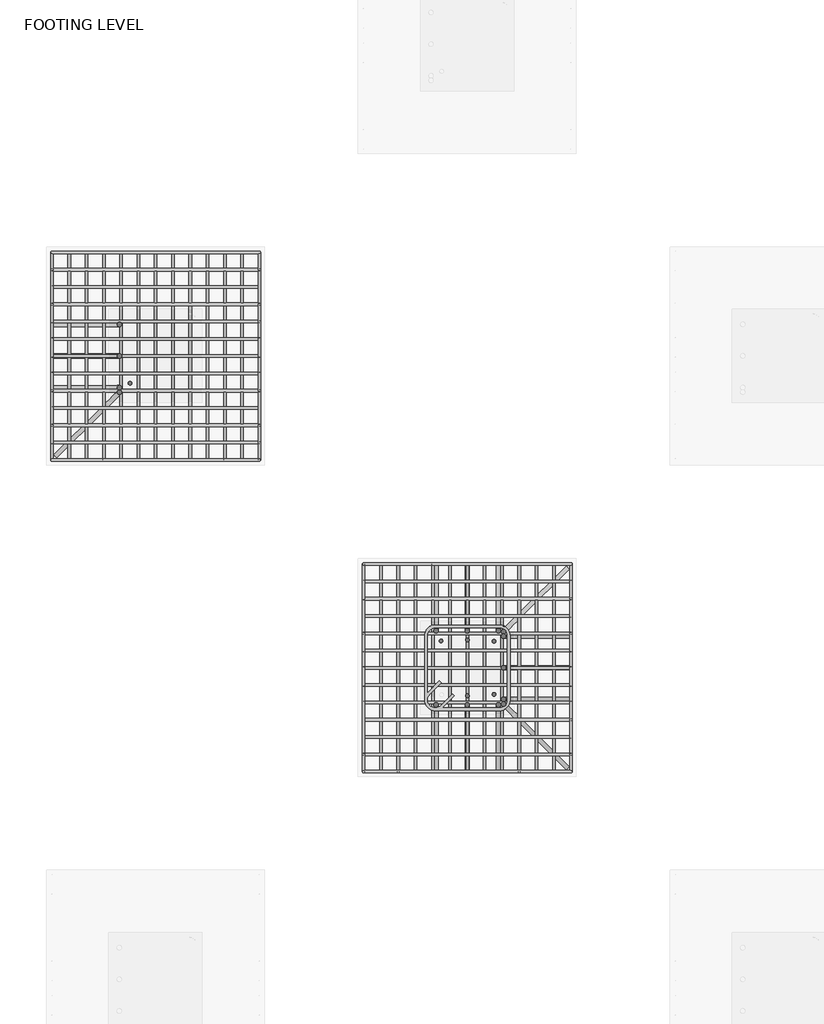
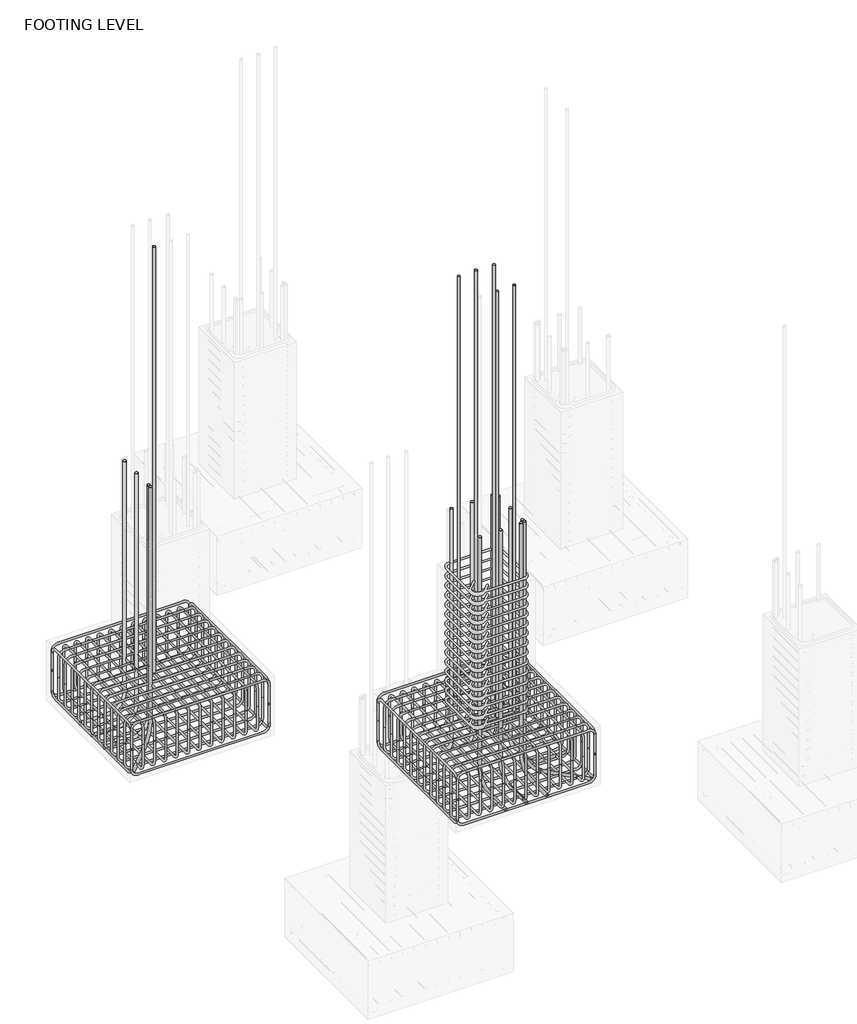
# One storey, part 4 of 10: 23 reinforcing bars.
"""IFC4 building model written with IfcOpenShell, lengths in millimetres."""

from ifc_helpers import new_model, si_unit, point, frame, origin, place, context, project, spatial, polyline, circle_curve, trimmed, segment, composite_curve, source, transform, mapped, element, save
from ifc_brep_helpers import swept_disk

model = new_model("IFC4")

# Units and contexts
model_context = context("Model", 3, world=origin())
ifc_project = project(units=[si_unit("LENGTHUNIT", "METRE", prefix="MILLI")], contexts=[model_context])

# Site, building, storey
site = spatial("IfcSite", under=ifc_project)
building = spatial("IfcBuilding", under=site)
storey = spatial("IfcBuildingStorey", under=building, Name="FOOTING LEVEL", Elevation=-2133.6)

# Reinforcing bars
placement = place(None, origin())
reinforcing_bar_shape = source(origin(), model_context, "Body", "SolidModel", [
    swept_disk(composite_curve([segment(polyline([(-11826.9269037, 6852.4829396, -2583.0), (-11826.9269037, 6852.4829396, -2905.1)]), True, "CONTINUOUS"), segment(trimmed(circle_curve(frame((-11917.1269037, 6852.4829396, -2905.1), z_axis=(0.0, 1.0, 0.0), x_axis=(90.20000000000073, 0.0, 0.0)), 90.2), [point((-11826.9269037, 6852.4829396, -2905.1))], [point((-11917.1269037, 6852.4829396, -2995.3))], True, "CARTESIAN"), True, "CONTINUOUS"), segment(polyline([(-11917.1269037, 6852.4829396, -2995.3), (-13764.9269037, 6852.4829396, -2995.3)]), True, "CONTINUOUS"), segment(trimmed(circle_curve(frame((-13764.9269037, 6852.4829396, -2905.1), z_axis=(0.0, 1.0, 0.0), x_axis=(0.0, 0.0, -90.20000000000027)), 90.2), [point((-13764.9269037, 6852.4829396, -2995.3))], [point((-13855.1269037, 6852.4829396, -2905.1))], True, "CARTESIAN"), True, "CONTINUOUS"), segment(polyline([(-13855.1269037, 6852.4829396, -2905.1), (-13855.1269037, 6852.4829396, -2583.0)]), True, "CONTINUOUS")], self_intersect=False), 12.7),
])
element("IfcReinforcingBar", 1, at=placement, inside=storey, context=model_context, shape_type="MappedRepresentation", body=[
    mapped(reinforcing_bar_shape, transform((0.0, 0.0, 0.0), x_axis=(1.0, 0.0, 0.0), y_axis=(0.0, 1.0, 0.0), z_axis=(0.0, 0.0, 1.0))),
    mapped(reinforcing_bar_shape, transform((0.0, -169.0166667, 0.0), x_axis=(1.0, 0.0, 0.0), y_axis=(0.0, 1.0, 0.0), z_axis=(0.0, 0.0, 1.0))),
    mapped(reinforcing_bar_shape, transform((0.0, -338.0333333, 0.0), x_axis=(1.0, 0.0, 0.0), y_axis=(0.0, 1.0, 0.0), z_axis=(0.0, 0.0, 1.0))),
    mapped(reinforcing_bar_shape, transform((0.0, -507.05, 0.0), x_axis=(1.0, 0.0, 0.0), y_axis=(0.0, 1.0, 0.0), z_axis=(0.0, 0.0, 1.0))),
    mapped(reinforcing_bar_shape, transform((0.0, -676.0666667, 0.0), x_axis=(1.0, 0.0, 0.0), y_axis=(0.0, 1.0, 0.0), z_axis=(0.0, 0.0, 1.0))),
    mapped(reinforcing_bar_shape, transform((0.0, -845.0833333, 0.0), x_axis=(1.0, 0.0, 0.0), y_axis=(0.0, 1.0, 0.0), z_axis=(0.0, 0.0, 1.0))),
    mapped(reinforcing_bar_shape, transform((0.0, -1014.1, 0.0), x_axis=(1.0, 0.0, 0.0), y_axis=(0.0, 1.0, 0.0), z_axis=(0.0, 0.0, 1.0))),
    mapped(reinforcing_bar_shape, transform((0.0, -1183.1166667, 0.0), x_axis=(1.0, 0.0, 0.0), y_axis=(0.0, 1.0, 0.0), z_axis=(0.0, 0.0, 1.0))),
    mapped(reinforcing_bar_shape, transform((0.0, -1352.1333333, 0.0), x_axis=(1.0, 0.0, 0.0), y_axis=(0.0, 1.0, 0.0), z_axis=(0.0, 0.0, 1.0))),
    mapped(reinforcing_bar_shape, transform((0.0, -1521.15, 0.0), x_axis=(1.0, 0.0, 0.0), y_axis=(0.0, 1.0, 0.0), z_axis=(0.0, 0.0, 1.0))),
    mapped(reinforcing_bar_shape, transform((0.0, -1690.1666667, 0.0), x_axis=(1.0, 0.0, 0.0), y_axis=(0.0, 1.0, 0.0), z_axis=(0.0, 0.0, 1.0))),
    mapped(reinforcing_bar_shape, transform((0.0, -1859.1833333, 0.0), x_axis=(1.0, 0.0, 0.0), y_axis=(0.0, 1.0, 0.0), z_axis=(0.0, 0.0, 1.0))),
    mapped(reinforcing_bar_shape, transform((0.0, -2028.2, 0.0), x_axis=(1.0, 0.0, 0.0), y_axis=(0.0, 1.0, 0.0), z_axis=(0.0, 0.0, 1.0))),
])
reinforcing_bar_2_shape = source(origin(), model_context, "Body", "SolidModel", [
    swept_disk(composite_curve([segment(polyline([(-13855.1269037, 6852.4829396, -2598.6), (-13855.1269037, 6852.4829396, -2276.5)]), True, "CONTINUOUS"), segment(trimmed(circle_curve(frame((-13764.9269037, 6852.4829396, -2276.5), z_axis=(0.0, 1.0, 0.0), x_axis=(-90.20000000000073, 0.0, 0.0)), 90.2), [point((-13855.1269037, 6852.4829396, -2276.5))], [point((-13764.9269037, 6852.4829396, -2186.3))], True, "CARTESIAN"), True, "CONTINUOUS"), segment(polyline([(-13764.9269037, 6852.4829396, -2186.3), (-11917.1269037, 6852.4829396, -2186.3)]), True, "CONTINUOUS"), segment(trimmed(circle_curve(frame((-11917.1269037, 6852.4829396, -2276.5), z_axis=(0.0, 1.0, 0.0), x_axis=(0.0, 0.0, 90.19999999999982)), 90.2), [point((-11917.1269037, 6852.4829396, -2186.3))], [point((-11826.9269037, 6852.4829396, -2276.5))], True, "CARTESIAN"), True, "CONTINUOUS"), segment(polyline([(-11826.9269037, 6852.4829396, -2276.5), (-11826.9269037, 6852.4829396, -2598.6)]), True, "CONTINUOUS")], self_intersect=False), 12.7),
])
element("IfcReinforcingBar", 2, at=placement, inside=storey, context=model_context, shape_type="MappedRepresentation", body=[
    mapped(reinforcing_bar_2_shape, transform((0.0, 0.0, 0.0), x_axis=(1.0, 0.0, 0.0), y_axis=(0.0, 1.0, 0.0), z_axis=(0.0, 0.0, 1.0))),
    mapped(reinforcing_bar_2_shape, transform((0.0, -169.0166667, 0.0), x_axis=(1.0, 0.0, 0.0), y_axis=(0.0, 1.0, 0.0), z_axis=(0.0, 0.0, 1.0))),
    mapped(reinforcing_bar_2_shape, transform((0.0, -338.0333333, 0.0), x_axis=(1.0, 0.0, 0.0), y_axis=(0.0, 1.0, 0.0), z_axis=(0.0, 0.0, 1.0))),
    mapped(reinforcing_bar_2_shape, transform((0.0, -507.05, 0.0), x_axis=(1.0, 0.0, 0.0), y_axis=(0.0, 1.0, 0.0), z_axis=(0.0, 0.0, 1.0))),
    mapped(reinforcing_bar_2_shape, transform((0.0, -676.0666667, 0.0), x_axis=(1.0, 0.0, 0.0), y_axis=(0.0, 1.0, 0.0), z_axis=(0.0, 0.0, 1.0))),
    mapped(reinforcing_bar_2_shape, transform((0.0, -845.0833333, 0.0), x_axis=(1.0, 0.0, 0.0), y_axis=(0.0, 1.0, 0.0), z_axis=(0.0, 0.0, 1.0))),
    mapped(reinforcing_bar_2_shape, transform((0.0, -1014.1, 0.0), x_axis=(1.0, 0.0, 0.0), y_axis=(0.0, 1.0, 0.0), z_axis=(0.0, 0.0, 1.0))),
    mapped(reinforcing_bar_2_shape, transform((0.0, -1183.1166667, 0.0), x_axis=(1.0, 0.0, 0.0), y_axis=(0.0, 1.0, 0.0), z_axis=(0.0, 0.0, 1.0))),
    mapped(reinforcing_bar_2_shape, transform((0.0, -1352.1333333, 0.0), x_axis=(1.0, 0.0, 0.0), y_axis=(0.0, 1.0, 0.0), z_axis=(0.0, 0.0, 1.0))),
    mapped(reinforcing_bar_2_shape, transform((0.0, -1521.15, 0.0), x_axis=(1.0, 0.0, 0.0), y_axis=(0.0, 1.0, 0.0), z_axis=(0.0, 0.0, 1.0))),
    mapped(reinforcing_bar_2_shape, transform((0.0, -1690.1666667, 0.0), x_axis=(1.0, 0.0, 0.0), y_axis=(0.0, 1.0, 0.0), z_axis=(0.0, 0.0, 1.0))),
    mapped(reinforcing_bar_2_shape, transform((0.0, -1859.1833333, 0.0), x_axis=(1.0, 0.0, 0.0), y_axis=(0.0, 1.0, 0.0), z_axis=(0.0, 0.0, 1.0))),
    mapped(reinforcing_bar_2_shape, transform((0.0, -2028.2, 0.0), x_axis=(1.0, 0.0, 0.0), y_axis=(0.0, 1.0, 0.0), z_axis=(0.0, 0.0, 1.0))),
])
reinforcing_bar_3_shape = source(origin(), model_context, "Body", "SolidModel", [
    swept_disk(composite_curve([segment(polyline([(-11826.9269037, 4824.2829396, -2559.4978077), (-11826.9269037, 4824.2829396, -2881.5978077)]), True, "CONTINUOUS"), segment(trimmed(circle_curve(frame((-11826.9269037, 4914.4829396, -2881.5978077), z_axis=(1.0, 0.0, 0.0), x_axis=(0.0, -90.19999999999982, 0.0)), 90.2), [point((-11826.9269037, 4824.2829396, -2881.5978077))], [point((-11826.9269037, 4914.4829396, -2971.7978077))], True, "CARTESIAN"), True, "CONTINUOUS"), segment(polyline([(-11826.9269037, 4914.4829396, -2971.7978077), (-11826.9269037, 6762.2829396, -2971.7978077)]), True, "CONTINUOUS"), segment(trimmed(circle_curve(frame((-11826.9269037, 6762.2829396, -2881.5978077), z_axis=(1.0, 0.0, 0.0), x_axis=(0.0, 0.0, -90.19999999999982)), 90.2), [point((-11826.9269037, 6762.2829396, -2971.7978077))], [point((-11826.9269037, 6852.4829396, -2881.5978077))], True, "CARTESIAN"), True, "CONTINUOUS"), segment(polyline([(-11826.9269037, 6852.4829396, -2881.5978077), (-11826.9269037, 6852.4829396, -2559.4978077)]), True, "CONTINUOUS")], self_intersect=False), 12.7),
])
element("IfcReinforcingBar", 3, at=placement, inside=storey, context=model_context, shape_type="MappedRepresentation", body=[
    mapped(reinforcing_bar_3_shape, transform((0.0, 0.0, 0.0), x_axis=(1.0, 0.0, 0.0), y_axis=(0.0, 1.0, 0.0), z_axis=(0.0, 0.0, 1.0))),
    mapped(reinforcing_bar_3_shape, transform((-169.0166667, 0.0, 0.0), x_axis=(1.0, 0.0, 0.0), y_axis=(0.0, 1.0, 0.0), z_axis=(0.0, 0.0, 1.0))),
    mapped(reinforcing_bar_3_shape, transform((-338.0333333, 0.0, 0.0), x_axis=(1.0, 0.0, 0.0), y_axis=(0.0, 1.0, 0.0), z_axis=(0.0, 0.0, 1.0))),
    mapped(reinforcing_bar_3_shape, transform((-507.05, 0.0, 0.0), x_axis=(1.0, 0.0, 0.0), y_axis=(0.0, 1.0, 0.0), z_axis=(0.0, 0.0, 1.0))),
    mapped(reinforcing_bar_3_shape, transform((-676.0666667, 0.0, 0.0), x_axis=(1.0, 0.0, 0.0), y_axis=(0.0, 1.0, 0.0), z_axis=(0.0, 0.0, 1.0))),
    mapped(reinforcing_bar_3_shape, transform((-845.0833333, 0.0, 0.0), x_axis=(1.0, 0.0, 0.0), y_axis=(0.0, 1.0, 0.0), z_axis=(0.0, 0.0, 1.0))),
    mapped(reinforcing_bar_3_shape, transform((-1014.1, 0.0, 0.0), x_axis=(1.0, 0.0, 0.0), y_axis=(0.0, 1.0, 0.0), z_axis=(0.0, 0.0, 1.0))),
    mapped(reinforcing_bar_3_shape, transform((-1183.1166667, 0.0, 0.0), x_axis=(1.0, 0.0, 0.0), y_axis=(0.0, 1.0, 0.0), z_axis=(0.0, 0.0, 1.0))),
    mapped(reinforcing_bar_3_shape, transform((-1352.1333333, 0.0, 0.0), x_axis=(1.0, 0.0, 0.0), y_axis=(0.0, 1.0, 0.0), z_axis=(0.0, 0.0, 1.0))),
    mapped(reinforcing_bar_3_shape, transform((-1521.15, 0.0, 0.0), x_axis=(1.0, 0.0, 0.0), y_axis=(0.0, 1.0, 0.0), z_axis=(0.0, 0.0, 1.0))),
    mapped(reinforcing_bar_3_shape, transform((-1690.1666667, 0.0, 0.0), x_axis=(1.0, 0.0, 0.0), y_axis=(0.0, 1.0, 0.0), z_axis=(0.0, 0.0, 1.0))),
    mapped(reinforcing_bar_3_shape, transform((-1859.1833333, 0.0, 0.0), x_axis=(1.0, 0.0, 0.0), y_axis=(0.0, 1.0, 0.0), z_axis=(0.0, 0.0, 1.0))),
    mapped(reinforcing_bar_3_shape, transform((-2028.2, 0.0, 0.0), x_axis=(1.0, 0.0, 0.0), y_axis=(0.0, 1.0, 0.0), z_axis=(0.0, 0.0, 1.0))),
])
reinforcing_bar_4_shape = source(origin(), model_context, "Body", "SolidModel", [
    swept_disk(composite_curve([segment(polyline([(-13855.1269037, 4824.2829396, -2622.9919875), (-13855.1269037, 4824.2829396, -2300.8919875)]), True, "CONTINUOUS"), segment(trimmed(circle_curve(frame((-13855.1269037, 4914.4829396, -2300.8919875), z_axis=(-1.0, 0.0, 0.0), x_axis=(0.0, -90.19999999999982, 0.0)), 90.2), [point((-13855.1269037, 4824.2829396, -2300.8919875))], [point((-13855.1269037, 4914.4829396, -2210.6919875))], True, "CARTESIAN"), True, "CONTINUOUS"), segment(polyline([(-13855.1269037, 4914.4829396, -2210.6919875), (-13855.1269037, 6762.2829396, -2210.6919875)]), True, "CONTINUOUS"), segment(trimmed(circle_curve(frame((-13855.1269037, 6762.2829396, -2300.8919875), z_axis=(-1.0, 0.0, 0.0), x_axis=(0.0, 0.0, 90.20000000000027)), 90.2), [point((-13855.1269037, 6762.2829396, -2210.6919875))], [point((-13855.1269037, 6852.4829396, -2300.8919875))], True, "CARTESIAN"), True, "CONTINUOUS"), segment(polyline([(-13855.1269037, 6852.4829396, -2300.8919875), (-13855.1269037, 6852.4829396, -2622.9919875)]), True, "CONTINUOUS")], self_intersect=False), 12.7),
])
element("IfcReinforcingBar", 4, at=placement, inside=storey, context=model_context, shape_type="MappedRepresentation", body=[
    mapped(reinforcing_bar_4_shape, transform((0.0, 0.0, 0.0), x_axis=(1.0, 0.0, 0.0), y_axis=(0.0, 1.0, 0.0), z_axis=(0.0, 0.0, 1.0))),
    mapped(reinforcing_bar_4_shape, transform((169.0166667, 0.0, 0.0), x_axis=(1.0, 0.0, 0.0), y_axis=(0.0, 1.0, 0.0), z_axis=(0.0, 0.0, 1.0))),
    mapped(reinforcing_bar_4_shape, transform((338.0333333, 0.0, 0.0), x_axis=(1.0, 0.0, 0.0), y_axis=(0.0, 1.0, 0.0), z_axis=(0.0, 0.0, 1.0))),
    mapped(reinforcing_bar_4_shape, transform((507.05, 0.0, 0.0), x_axis=(1.0, 0.0, 0.0), y_axis=(0.0, 1.0, 0.0), z_axis=(0.0, 0.0, 1.0))),
    mapped(reinforcing_bar_4_shape, transform((676.0666667, 0.0, 0.0), x_axis=(1.0, 0.0, 0.0), y_axis=(0.0, 1.0, 0.0), z_axis=(0.0, 0.0, 1.0))),
    mapped(reinforcing_bar_4_shape, transform((845.0833333, 0.0, 0.0), x_axis=(1.0, 0.0, 0.0), y_axis=(0.0, 1.0, 0.0), z_axis=(0.0, 0.0, 1.0))),
    mapped(reinforcing_bar_4_shape, transform((1014.1, 0.0, 0.0), x_axis=(1.0, 0.0, 0.0), y_axis=(0.0, 1.0, 0.0), z_axis=(0.0, 0.0, 1.0))),
    mapped(reinforcing_bar_4_shape, transform((1183.1166667, 0.0, 0.0), x_axis=(1.0, 0.0, 0.0), y_axis=(0.0, 1.0, 0.0), z_axis=(0.0, 0.0, 1.0))),
    mapped(reinforcing_bar_4_shape, transform((1352.1333333, 0.0, 0.0), x_axis=(1.0, 0.0, 0.0), y_axis=(0.0, 1.0, 0.0), z_axis=(0.0, 0.0, 1.0))),
    mapped(reinforcing_bar_4_shape, transform((1521.15, 0.0, 0.0), x_axis=(1.0, 0.0, 0.0), y_axis=(0.0, 1.0, 0.0), z_axis=(0.0, 0.0, 1.0))),
    mapped(reinforcing_bar_4_shape, transform((1690.1666667, 0.0, 0.0), x_axis=(1.0, 0.0, 0.0), y_axis=(0.0, 1.0, 0.0), z_axis=(0.0, 0.0, 1.0))),
    mapped(reinforcing_bar_4_shape, transform((1859.1833333, 0.0, 0.0), x_axis=(1.0, 0.0, 0.0), y_axis=(0.0, 1.0, 0.0), z_axis=(0.0, 0.0, 1.0))),
    mapped(reinforcing_bar_4_shape, transform((2028.2, 0.0, 0.0), x_axis=(1.0, 0.0, 0.0), y_axis=(0.0, 1.0, 0.0), z_axis=(0.0, 0.0, 1.0))),
])
reinforcing_bar_5_shape = source(origin(), model_context, "Body", "SolidModel", [
    swept_disk(composite_curve([segment(polyline([(-8778.9269037, 3804.4829396, -2583.0), (-8778.9269037, 3804.4829396, -2905.1)]), True, "CONTINUOUS"), segment(trimmed(circle_curve(frame((-8869.1269037, 3804.4829396, -2905.1), z_axis=(0.0, 1.0, 0.0), x_axis=(90.20000000000073, 0.0, 0.0)), 90.2), [point((-8778.9269037, 3804.4829396, -2905.1))], [point((-8869.1269037, 3804.4829396, -2995.3))], True, "CARTESIAN"), True, "CONTINUOUS"), segment(polyline([(-8869.1269037, 3804.4829396, -2995.3), (-10716.9269037, 3804.4829396, -2995.3)]), True, "CONTINUOUS"), segment(trimmed(circle_curve(frame((-10716.9269037, 3804.4829396, -2905.1), z_axis=(0.0, 1.0, 0.0), x_axis=(0.0, 0.0, -90.20000000000027)), 90.2), [point((-10716.9269037, 3804.4829396, -2995.3))], [point((-10807.1269037, 3804.4829396, -2905.1))], True, "CARTESIAN"), True, "CONTINUOUS"), segment(polyline([(-10807.1269037, 3804.4829396, -2905.1), (-10807.1269037, 3804.4829396, -2583.0)]), True, "CONTINUOUS")], self_intersect=False), 12.7),
])
element("IfcReinforcingBar", 5, at=placement, inside=storey, context=model_context, shape_type="MappedRepresentation", body=[
    mapped(reinforcing_bar_5_shape, transform((0.0, 0.0, 0.0), x_axis=(1.0, 0.0, 0.0), y_axis=(0.0, 1.0, 0.0), z_axis=(0.0, 0.0, 1.0))),
    mapped(reinforcing_bar_5_shape, transform((0.0, -169.0166667, 0.0), x_axis=(1.0, 0.0, 0.0), y_axis=(0.0, 1.0, 0.0), z_axis=(0.0, 0.0, 1.0))),
    mapped(reinforcing_bar_5_shape, transform((0.0, -338.0333333, 0.0), x_axis=(1.0, 0.0, 0.0), y_axis=(0.0, 1.0, 0.0), z_axis=(0.0, 0.0, 1.0))),
    mapped(reinforcing_bar_5_shape, transform((0.0, -507.05, 0.0), x_axis=(1.0, 0.0, 0.0), y_axis=(0.0, 1.0, 0.0), z_axis=(0.0, 0.0, 1.0))),
    mapped(reinforcing_bar_5_shape, transform((0.0, -676.0666667, 0.0), x_axis=(1.0, 0.0, 0.0), y_axis=(0.0, 1.0, 0.0), z_axis=(0.0, 0.0, 1.0))),
    mapped(reinforcing_bar_5_shape, transform((0.0, -845.0833333, 0.0), x_axis=(1.0, 0.0, 0.0), y_axis=(0.0, 1.0, 0.0), z_axis=(0.0, 0.0, 1.0))),
    mapped(reinforcing_bar_5_shape, transform((0.0, -1014.1, 0.0), x_axis=(1.0, 0.0, 0.0), y_axis=(0.0, 1.0, 0.0), z_axis=(0.0, 0.0, 1.0))),
    mapped(reinforcing_bar_5_shape, transform((0.0, -1183.1166667, 0.0), x_axis=(1.0, 0.0, 0.0), y_axis=(0.0, 1.0, 0.0), z_axis=(0.0, 0.0, 1.0))),
    mapped(reinforcing_bar_5_shape, transform((0.0, -1352.1333333, 0.0), x_axis=(1.0, 0.0, 0.0), y_axis=(0.0, 1.0, 0.0), z_axis=(0.0, 0.0, 1.0))),
    mapped(reinforcing_bar_5_shape, transform((0.0, -1521.15, 0.0), x_axis=(1.0, 0.0, 0.0), y_axis=(0.0, 1.0, 0.0), z_axis=(0.0, 0.0, 1.0))),
    mapped(reinforcing_bar_5_shape, transform((0.0, -1690.1666667, 0.0), x_axis=(1.0, 0.0, 0.0), y_axis=(0.0, 1.0, 0.0), z_axis=(0.0, 0.0, 1.0))),
    mapped(reinforcing_bar_5_shape, transform((0.0, -1859.1833333, 0.0), x_axis=(1.0, 0.0, 0.0), y_axis=(0.0, 1.0, 0.0), z_axis=(0.0, 0.0, 1.0))),
    mapped(reinforcing_bar_5_shape, transform((0.0, -2028.2, 0.0), x_axis=(1.0, 0.0, 0.0), y_axis=(0.0, 1.0, 0.0), z_axis=(0.0, 0.0, 1.0))),
])
reinforcing_bar_6_shape = source(origin(), model_context, "Body", "SolidModel", [
    swept_disk(composite_curve([segment(polyline([(-10807.1269037, 3804.4829396, -2598.6), (-10807.1269037, 3804.4829396, -2276.5)]), True, "CONTINUOUS"), segment(trimmed(circle_curve(frame((-10716.9269037, 3804.4829396, -2276.5), z_axis=(0.0, 1.0, 0.0), x_axis=(-90.20000000000073, 0.0, 0.0)), 90.2), [point((-10807.1269037, 3804.4829396, -2276.5))], [point((-10716.9269037, 3804.4829396, -2186.3))], True, "CARTESIAN"), True, "CONTINUOUS"), segment(polyline([(-10716.9269037, 3804.4829396, -2186.3), (-8869.1269037, 3804.4829396, -2186.3)]), True, "CONTINUOUS"), segment(trimmed(circle_curve(frame((-8869.1269037, 3804.4829396, -2276.5), z_axis=(0.0, 1.0, 0.0), x_axis=(0.0, 0.0, 90.19999999999982)), 90.2), [point((-8869.1269037, 3804.4829396, -2186.3))], [point((-8778.9269037, 3804.4829396, -2276.5))], True, "CARTESIAN"), True, "CONTINUOUS"), segment(polyline([(-8778.9269037, 3804.4829396, -2276.5), (-8778.9269037, 3804.4829396, -2598.6)]), True, "CONTINUOUS")], self_intersect=False), 12.7),
])
element("IfcReinforcingBar", 6, at=placement, inside=storey, context=model_context, shape_type="MappedRepresentation", body=[
    mapped(reinforcing_bar_6_shape, transform((0.0, 0.0, 0.0), x_axis=(1.0, 0.0, 0.0), y_axis=(0.0, 1.0, 0.0), z_axis=(0.0, 0.0, 1.0))),
    mapped(reinforcing_bar_6_shape, transform((0.0, -169.0166667, 0.0), x_axis=(1.0, 0.0, 0.0), y_axis=(0.0, 1.0, 0.0), z_axis=(0.0, 0.0, 1.0))),
    mapped(reinforcing_bar_6_shape, transform((0.0, -338.0333333, 0.0), x_axis=(1.0, 0.0, 0.0), y_axis=(0.0, 1.0, 0.0), z_axis=(0.0, 0.0, 1.0))),
    mapped(reinforcing_bar_6_shape, transform((0.0, -507.05, 0.0), x_axis=(1.0, 0.0, 0.0), y_axis=(0.0, 1.0, 0.0), z_axis=(0.0, 0.0, 1.0))),
    mapped(reinforcing_bar_6_shape, transform((0.0, -676.0666667, 0.0), x_axis=(1.0, 0.0, 0.0), y_axis=(0.0, 1.0, 0.0), z_axis=(0.0, 0.0, 1.0))),
    mapped(reinforcing_bar_6_shape, transform((0.0, -845.0833333, 0.0), x_axis=(1.0, 0.0, 0.0), y_axis=(0.0, 1.0, 0.0), z_axis=(0.0, 0.0, 1.0))),
    mapped(reinforcing_bar_6_shape, transform((0.0, -1014.1, 0.0), x_axis=(1.0, 0.0, 0.0), y_axis=(0.0, 1.0, 0.0), z_axis=(0.0, 0.0, 1.0))),
    mapped(reinforcing_bar_6_shape, transform((0.0, -1183.1166667, 0.0), x_axis=(1.0, 0.0, 0.0), y_axis=(0.0, 1.0, 0.0), z_axis=(0.0, 0.0, 1.0))),
    mapped(reinforcing_bar_6_shape, transform((0.0, -1352.1333333, 0.0), x_axis=(1.0, 0.0, 0.0), y_axis=(0.0, 1.0, 0.0), z_axis=(0.0, 0.0, 1.0))),
    mapped(reinforcing_bar_6_shape, transform((0.0, -1521.15, 0.0), x_axis=(1.0, 0.0, 0.0), y_axis=(0.0, 1.0, 0.0), z_axis=(0.0, 0.0, 1.0))),
    mapped(reinforcing_bar_6_shape, transform((0.0, -1690.1666667, 0.0), x_axis=(1.0, 0.0, 0.0), y_axis=(0.0, 1.0, 0.0), z_axis=(0.0, 0.0, 1.0))),
    mapped(reinforcing_bar_6_shape, transform((0.0, -1859.1833333, 0.0), x_axis=(1.0, 0.0, 0.0), y_axis=(0.0, 1.0, 0.0), z_axis=(0.0, 0.0, 1.0))),
    mapped(reinforcing_bar_6_shape, transform((0.0, -2028.2, 0.0), x_axis=(1.0, 0.0, 0.0), y_axis=(0.0, 1.0, 0.0), z_axis=(0.0, 0.0, 1.0))),
])
reinforcing_bar_7_shape = source(origin(), model_context, "Body", "SolidModel", [
    swept_disk(composite_curve([segment(polyline([(-8778.9269037, 1776.2829396, -2559.4978077), (-8778.9269037, 1776.2829396, -2881.5978077)]), True, "CONTINUOUS"), segment(trimmed(circle_curve(frame((-8778.9269037, 1866.4829396, -2881.5978077), z_axis=(1.0, 0.0, 0.0), x_axis=(0.0, -90.20000000000005, 0.0)), 90.2), [point((-8778.9269037, 1776.2829396, -2881.5978077))], [point((-8778.9269037, 1866.4829396, -2971.7978077))], True, "CARTESIAN"), True, "CONTINUOUS"), segment(polyline([(-8778.9269037, 1866.4829396, -2971.7978077), (-8778.9269037, 3714.2829396, -2971.7978077)]), True, "CONTINUOUS"), segment(trimmed(circle_curve(frame((-8778.9269037, 3714.2829396, -2881.5978077), z_axis=(1.0, 0.0, 0.0), x_axis=(0.0, 0.0, -90.19999999999982)), 90.2), [point((-8778.9269037, 3714.2829396, -2971.7978077))], [point((-8778.9269037, 3804.4829396, -2881.5978077))], True, "CARTESIAN"), True, "CONTINUOUS"), segment(polyline([(-8778.9269037, 3804.4829396, -2881.5978077), (-8778.9269037, 3804.4829396, -2559.4978077)]), True, "CONTINUOUS")], self_intersect=False), 12.7),
])
element("IfcReinforcingBar", 7, at=placement, inside=storey, context=model_context, shape_type="MappedRepresentation", body=[
    mapped(reinforcing_bar_7_shape, transform((0.0, 0.0, 0.0), x_axis=(1.0, 0.0, 0.0), y_axis=(0.0, 1.0, 0.0), z_axis=(0.0, 0.0, 1.0))),
    mapped(reinforcing_bar_7_shape, transform((-169.0166667, 0.0, 0.0), x_axis=(1.0, 0.0, 0.0), y_axis=(0.0, 1.0, 0.0), z_axis=(0.0, 0.0, 1.0))),
    mapped(reinforcing_bar_7_shape, transform((-338.0333333, 0.0, 0.0), x_axis=(1.0, 0.0, 0.0), y_axis=(0.0, 1.0, 0.0), z_axis=(0.0, 0.0, 1.0))),
    mapped(reinforcing_bar_7_shape, transform((-507.05, 0.0, 0.0), x_axis=(1.0, 0.0, 0.0), y_axis=(0.0, 1.0, 0.0), z_axis=(0.0, 0.0, 1.0))),
    mapped(reinforcing_bar_7_shape, transform((-676.0666667, 0.0, 0.0), x_axis=(1.0, 0.0, 0.0), y_axis=(0.0, 1.0, 0.0), z_axis=(0.0, 0.0, 1.0))),
    mapped(reinforcing_bar_7_shape, transform((-845.0833333, 0.0, 0.0), x_axis=(1.0, 0.0, 0.0), y_axis=(0.0, 1.0, 0.0), z_axis=(0.0, 0.0, 1.0))),
    mapped(reinforcing_bar_7_shape, transform((-1014.1, 0.0, 0.0), x_axis=(1.0, 0.0, 0.0), y_axis=(0.0, 1.0, 0.0), z_axis=(0.0, 0.0, 1.0))),
    mapped(reinforcing_bar_7_shape, transform((-1183.1166667, 0.0, 0.0), x_axis=(1.0, 0.0, 0.0), y_axis=(0.0, 1.0, 0.0), z_axis=(0.0, 0.0, 1.0))),
    mapped(reinforcing_bar_7_shape, transform((-1352.1333333, 0.0, 0.0), x_axis=(1.0, 0.0, 0.0), y_axis=(0.0, 1.0, 0.0), z_axis=(0.0, 0.0, 1.0))),
    mapped(reinforcing_bar_7_shape, transform((-1521.15, 0.0, 0.0), x_axis=(1.0, 0.0, 0.0), y_axis=(0.0, 1.0, 0.0), z_axis=(0.0, 0.0, 1.0))),
    mapped(reinforcing_bar_7_shape, transform((-1690.1666667, 0.0, 0.0), x_axis=(1.0, 0.0, 0.0), y_axis=(0.0, 1.0, 0.0), z_axis=(0.0, 0.0, 1.0))),
    mapped(reinforcing_bar_7_shape, transform((-1859.1833333, 0.0, 0.0), x_axis=(1.0, 0.0, 0.0), y_axis=(0.0, 1.0, 0.0), z_axis=(0.0, 0.0, 1.0))),
    mapped(reinforcing_bar_7_shape, transform((-2028.2, 0.0, 0.0), x_axis=(1.0, 0.0, 0.0), y_axis=(0.0, 1.0, 0.0), z_axis=(0.0, 0.0, 1.0))),
])
reinforcing_bar_8_shape = source(origin(), model_context, "Body", "SolidModel", [
    swept_disk(composite_curve([segment(polyline([(-10807.1269037, 1776.2829396, -2622.9919875), (-10807.1269037, 1776.2829396, -2300.8919875)]), True, "CONTINUOUS"), segment(trimmed(circle_curve(frame((-10807.1269037, 1866.4829396, -2300.8919875), z_axis=(-1.0, 0.0, 0.0), x_axis=(0.0, -90.20000000000005, 0.0)), 90.2), [point((-10807.1269037, 1776.2829396, -2300.8919875))], [point((-10807.1269037, 1866.4829396, -2210.6919875))], True, "CARTESIAN"), True, "CONTINUOUS"), segment(polyline([(-10807.1269037, 1866.4829396, -2210.6919875), (-10807.1269037, 3714.2829396, -2210.6919875)]), True, "CONTINUOUS"), segment(trimmed(circle_curve(frame((-10807.1269037, 3714.2829396, -2300.8919875), z_axis=(-1.0, 0.0, 0.0), x_axis=(0.0, 0.0, 90.20000000000027)), 90.2), [point((-10807.1269037, 3714.2829396, -2210.6919875))], [point((-10807.1269037, 3804.4829396, -2300.8919875))], True, "CARTESIAN"), True, "CONTINUOUS"), segment(polyline([(-10807.1269037, 3804.4829396, -2300.8919875), (-10807.1269037, 3804.4829396, -2622.9919875)]), True, "CONTINUOUS")], self_intersect=False), 12.7),
])
element("IfcReinforcingBar", 8, at=placement, inside=storey, context=model_context, shape_type="MappedRepresentation", body=[
    mapped(reinforcing_bar_8_shape, transform((0.0, 0.0, 0.0), x_axis=(1.0, 0.0, 0.0), y_axis=(0.0, 1.0, 0.0), z_axis=(0.0, 0.0, 1.0))),
    mapped(reinforcing_bar_8_shape, transform((169.0166667, 0.0, 0.0), x_axis=(1.0, 0.0, 0.0), y_axis=(0.0, 1.0, 0.0), z_axis=(0.0, 0.0, 1.0))),
    mapped(reinforcing_bar_8_shape, transform((338.0333333, 0.0, 0.0), x_axis=(1.0, 0.0, 0.0), y_axis=(0.0, 1.0, 0.0), z_axis=(0.0, 0.0, 1.0))),
    mapped(reinforcing_bar_8_shape, transform((507.05, 0.0, 0.0), x_axis=(1.0, 0.0, 0.0), y_axis=(0.0, 1.0, 0.0), z_axis=(0.0, 0.0, 1.0))),
    mapped(reinforcing_bar_8_shape, transform((676.0666667, 0.0, 0.0), x_axis=(1.0, 0.0, 0.0), y_axis=(0.0, 1.0, 0.0), z_axis=(0.0, 0.0, 1.0))),
    mapped(reinforcing_bar_8_shape, transform((845.0833333, 0.0, 0.0), x_axis=(1.0, 0.0, 0.0), y_axis=(0.0, 1.0, 0.0), z_axis=(0.0, 0.0, 1.0))),
    mapped(reinforcing_bar_8_shape, transform((1014.1, 0.0, 0.0), x_axis=(1.0, 0.0, 0.0), y_axis=(0.0, 1.0, 0.0), z_axis=(0.0, 0.0, 1.0))),
    mapped(reinforcing_bar_8_shape, transform((1183.1166667, 0.0, 0.0), x_axis=(1.0, 0.0, 0.0), y_axis=(0.0, 1.0, 0.0), z_axis=(0.0, 0.0, 1.0))),
    mapped(reinforcing_bar_8_shape, transform((1352.1333333, 0.0, 0.0), x_axis=(1.0, 0.0, 0.0), y_axis=(0.0, 1.0, 0.0), z_axis=(0.0, 0.0, 1.0))),
    mapped(reinforcing_bar_8_shape, transform((1521.15, 0.0, 0.0), x_axis=(1.0, 0.0, 0.0), y_axis=(0.0, 1.0, 0.0), z_axis=(0.0, 0.0, 1.0))),
    mapped(reinforcing_bar_8_shape, transform((1690.1666667, 0.0, 0.0), x_axis=(1.0, 0.0, 0.0), y_axis=(0.0, 1.0, 0.0), z_axis=(0.0, 0.0, 1.0))),
    mapped(reinforcing_bar_8_shape, transform((1859.1833333, 0.0, 0.0), x_axis=(1.0, 0.0, 0.0), y_axis=(0.0, 1.0, 0.0), z_axis=(0.0, 0.0, 1.0))),
    mapped(reinforcing_bar_8_shape, transform((2028.2, 0.0, 0.0), x_axis=(1.0, 0.0, 0.0), y_axis=(0.0, 1.0, 0.0), z_axis=(0.0, 0.0, 1.0))),
])
reinforcing_bar_9_shape = source(origin(), model_context, "Body", "SolidModel", [
    swept_disk(composite_curve([segment(polyline([(-9930.1462687, 2525.7015113, 0.0), (-10043.545872, 2412.3019079, 0.0)]), True, "CONTINUOUS"), segment(trimmed(circle_curve(frame((-10107.3269037, 2476.0829396, 0.0), z_axis=(0.0, 0.0, -1.0), x_axis=(63.78103169999849, -63.78103169999986, 0.0)), 90.2), [point((-10043.545872, 2412.3019079, 0.0))], [point((-10197.5269037, 2476.0829396, 0.0))], True, "CARTESIAN"), True, "CONTINUOUS"), segment(polyline([(-10197.5269037, 2476.0829396, 0.0), (-10197.5269037, 3104.6829396, 0.0)]), True, "CONTINUOUS"), segment(trimmed(circle_curve(frame((-10107.3269037, 3104.6829396, 0.0), z_axis=(0.0, 0.0, -1.0), x_axis=(-90.20000000000073, 0.0, 0.0)), 90.2), [point((-10197.5269037, 3104.6829396, 0.0))], [point((-10107.3269037, 3194.8829396, 0.0))], True, "CARTESIAN"), True, "CONTINUOUS"), segment(polyline([(-10107.3269037, 3194.8829396, 0.0), (-9478.7269037, 3194.8829396, 0.0)]), True, "CONTINUOUS"), segment(trimmed(circle_curve(frame((-9478.7269037, 3104.7273645, 2.8305953), z_axis=(0.0, -0.03138132276777647, -0.9995074850051623), x_axis=(0.0, 90.15557510000008, -2.8305953)), 90.2), [point((-9478.7269037, 3194.8829396, 0.0))], [point((-9388.5269037, 3104.7273645, 2.8305953))], True, "CARTESIAN"), True, "CONTINUOUS"), segment(polyline([(-9388.5269037, 3104.7273645, 2.8305953), (-9388.5269037, 2476.0385147, 22.5694047)]), True, "CONTINUOUS"), segment(trimmed(circle_curve(frame((-9478.7269037, 2476.0385147, 22.5694047), z_axis=(0.0, -0.03138132276777647, -0.9995074850051623), x_axis=(90.20000000000073, 0.0, 0.0)), 90.2), [point((-9388.5269037, 2476.0385147, 22.5694047))], [point((-9478.7269037, 2385.8829396, 25.4))], True, "CARTESIAN"), True, "CONTINUOUS"), segment(polyline([(-9478.7269037, 2385.8829396, 25.4), (-10107.3269037, 2385.8829396, 25.4)]), True, "CONTINUOUS"), segment(trimmed(circle_curve(frame((-10107.3269037, 2476.0829396, 25.4), z_axis=(0.0, 0.0, -1.0), x_axis=(0.0, -90.19999999999982, 0.0)), 90.2), [point((-10107.3269037, 2385.8829396, 25.4))], [point((-10171.1079353, 2539.8639713, 25.4))], True, "CARTESIAN"), True, "CONTINUOUS"), segment(polyline([(-10171.1079353, 2539.8639713, 25.4), (-10057.708332, 2653.2635746, 25.4)]), True, "CONTINUOUS")], self_intersect=False), 12.7),
])
element("IfcReinforcingBar", 9, at=placement, inside=storey, context=model_context, shape_type="MappedRepresentation", body=[
    mapped(reinforcing_bar_9_shape, transform((0.0, 0.0, 0.0), x_axis=(1.0, 0.0, 0.0), y_axis=(0.0, 1.0, 0.0), z_axis=(0.0, 0.0, 1.0))),
    mapped(reinforcing_bar_9_shape, transform((0.0, 0.0, -148.6357143), x_axis=(1.0, 0.0, 0.0), y_axis=(0.0, 1.0, 0.0), z_axis=(0.0, 0.0, 1.0))),
    mapped(reinforcing_bar_9_shape, transform((0.0, 0.0, -297.2714286), x_axis=(1.0, 0.0, 0.0), y_axis=(0.0, 1.0, 0.0), z_axis=(0.0, 0.0, 1.0))),
    mapped(reinforcing_bar_9_shape, transform((0.0, 0.0, -445.9071429), x_axis=(1.0, 0.0, 0.0), y_axis=(0.0, 1.0, 0.0), z_axis=(0.0, 0.0, 1.0))),
    mapped(reinforcing_bar_9_shape, transform((0.0, 0.0, -594.5428571), x_axis=(1.0, 0.0, 0.0), y_axis=(0.0, 1.0, 0.0), z_axis=(0.0, 0.0, 1.0))),
    mapped(reinforcing_bar_9_shape, transform((0.0, 0.0, -743.1785714), x_axis=(1.0, 0.0, 0.0), y_axis=(0.0, 1.0, 0.0), z_axis=(0.0, 0.0, 1.0))),
    mapped(reinforcing_bar_9_shape, transform((0.0, 0.0, -891.8142857), x_axis=(1.0, 0.0, 0.0), y_axis=(0.0, 1.0, 0.0), z_axis=(0.0, 0.0, 1.0))),
    mapped(reinforcing_bar_9_shape, transform((0.0, 0.0, -1040.45), x_axis=(1.0, 0.0, 0.0), y_axis=(0.0, 1.0, 0.0), z_axis=(0.0, 0.0, 1.0))),
    mapped(reinforcing_bar_9_shape, transform((0.0, 0.0, -1189.0857143), x_axis=(1.0, 0.0, 0.0), y_axis=(0.0, 1.0, 0.0), z_axis=(0.0, 0.0, 1.0))),
    mapped(reinforcing_bar_9_shape, transform((0.0, 0.0, -1337.7214286), x_axis=(1.0, 0.0, 0.0), y_axis=(0.0, 1.0, 0.0), z_axis=(0.0, 0.0, 1.0))),
    mapped(reinforcing_bar_9_shape, transform((0.0, 0.0, -1486.3571429), x_axis=(1.0, 0.0, 0.0), y_axis=(0.0, 1.0, 0.0), z_axis=(0.0, 0.0, 1.0))),
    mapped(reinforcing_bar_9_shape, transform((0.0, 0.0, -1634.9928571), x_axis=(1.0, 0.0, 0.0), y_axis=(0.0, 1.0, 0.0), z_axis=(0.0, 0.0, 1.0))),
    mapped(reinforcing_bar_9_shape, transform((0.0, 0.0, -1783.6285714), x_axis=(1.0, 0.0, 0.0), y_axis=(0.0, 1.0, 0.0), z_axis=(0.0, 0.0, 1.0))),
    mapped(reinforcing_bar_9_shape, transform((0.0, 0.0, -1932.2642857), x_axis=(1.0, 0.0, 0.0), y_axis=(0.0, 1.0, 0.0), z_axis=(0.0, 0.0, 1.0))),
    mapped(reinforcing_bar_9_shape, transform((0.0, 0.0, -2080.9), x_axis=(1.0, 0.0, 0.0), y_axis=(0.0, 1.0, 0.0), z_axis=(0.0, 0.0, 1.0))),
])
element("IfcReinforcingBar", 10, at=placement, inside=storey, context=model_context, shape_type="SolidModel", body=[
    swept_disk(composite_curve([segment(polyline([(-8812.5730107, 1809.9290467, -2976.5), (-9259.5238015, 2256.8798374, -2976.5)]), True, "CONTINUOUS"), segment(trimmed(circle_curve(frame((-9259.5238015, 2256.8798374, -2722.5), z_axis=(0.7071067811865508, 0.7071067811865444, 0.0), x_axis=(0.0, 0.0, -254.0)), 254.0), [point((-9259.5238015, 2256.8798374, -2976.5))], [point((-9439.1289239, 2436.4849599, -2722.5))], True, "CARTESIAN"), True, "CONTINUOUS"), segment(polyline([(-9439.1289239, 2436.4849599, -2722.5), (-9439.1289239, 2436.4849599, 874.4)]), True, "CONTINUOUS")], self_intersect=False), 21.5),
])
element("IfcReinforcingBar", 11, at=placement, inside=storey, context=model_context, shape_type="SolidModel", body=[
    swept_disk(composite_curve([segment(polyline([(-8812.5730107, 3770.8368325, -2976.5), (-9259.5238015, 3323.8860418, -2976.5)]), True, "CONTINUOUS"), segment(trimmed(circle_curve(frame((-9259.5238015, 3323.8860418, -2722.5), z_axis=(-0.7071067811865475, 0.7071067811865477, 0.0), x_axis=(0.0, 0.0, -254.0)), 254.0), [point((-9259.5238015, 3323.8860418, -2976.5))], [point((-9439.1289239, 3144.2809193, -2722.5))], True, "CARTESIAN"), True, "CONTINUOUS"), segment(polyline([(-9439.1289239, 3144.2809193, -2722.5), (-9439.1289239, 3144.2809193, 874.4)]), True, "CONTINUOUS")], self_intersect=False), 21.5),
])
element("IfcReinforcingBar", 12, at=placement, inside=storey, context=model_context, shape_type="SolidModel", body=[
    swept_disk(composite_curve([segment(polyline([(-8812.5730107, 1809.9290467, -2976.5), (-9259.5238015, 2256.8798374, -2976.5)]), True, "CONTINUOUS"), segment(trimmed(circle_curve(frame((-9259.5238015, 2256.8798374, -2722.5), z_axis=(0.7071067811865508, 0.7071067811865444, 0.0), x_axis=(0.0, 0.0, -254.0)), 254.0), [point((-9259.5238015, 2256.8798374, -2976.5))], [point((-9439.1289239, 2436.4849599, -2722.5))], True, "CARTESIAN"), True, "CONTINUOUS"), segment(polyline([(-9439.1289239, 2436.4849599, -2722.5), (-9439.1289239, 2436.4849599, 874.4)]), True, "CONTINUOUS")], self_intersect=False), 21.5),
])
reinforcing_bar_10_shape = source(origin(), model_context, "Body", "SolidModel", [
    swept_disk(composite_curve([segment(polyline([(-8776.2269037, 2482.0019966, -2976.5), (-9185.1289239, 2482.0019966, -2976.5)]), True, "CONTINUOUS"), segment(trimmed(circle_curve(frame((-9185.1289239, 2482.0019966, -2722.5), z_axis=(0.0, 1.0, 0.0), x_axis=(0.0, 0.0, -254.0)), 254.0), [point((-9185.1289239, 2482.0019966, -2976.5))], [point((-9439.1289239, 2482.0019966, -2722.5))], True, "CARTESIAN"), True, "CONTINUOUS"), segment(polyline([(-9439.1289239, 2482.0019966, -2722.5), (-9439.1289239, 2482.0019966, 874.4)]), True, "CONTINUOUS")], self_intersect=False), 21.5),
])
element("IfcReinforcingBar", 13, at=placement, inside=storey, context=model_context, shape_type="MappedRepresentation", body=[
    mapped(reinforcing_bar_10_shape, transform((0.0, 0.0, 0.0), x_axis=(1.0, 0.0, 0.0), y_axis=(0.0, 1.0, 0.0), z_axis=(0.0, 0.0, 1.0))),
    mapped(reinforcing_bar_10_shape, transform((0.0, 309.128507, 0.0), x_axis=(1.0, 0.0, 0.0), y_axis=(0.0, 1.0, 0.0), z_axis=(0.0, 0.0, 1.0))),
    mapped(reinforcing_bar_10_shape, transform((0.0, 618.2570139, 0.0), x_axis=(1.0, 0.0, 0.0), y_axis=(0.0, 1.0, 0.0), z_axis=(0.0, 0.0, 1.0))),
])
reinforcing_bar_11_shape = source(origin(), model_context, "Body", "SolidModel", [
    swept_disk(composite_curve([segment(polyline([(-9489.6587573, 3815.4257505, -2976.5), (-9489.6587573, 3406.5237302, -2976.5)]), True, "CONTINUOUS"), segment(trimmed(circle_curve(frame((-9489.6587573, 3406.5237302, -2722.5), z_axis=(-1.0, 0.0, 0.0), x_axis=(0.0, 0.0, -254.0)), 254.0), [point((-9489.6587573, 3406.5237302, -2976.5))], [point((-9489.6587573, 3152.5237302, -2722.5))], True, "CARTESIAN"), True, "CONTINUOUS"), segment(polyline([(-9489.6587573, 3152.5237302, -2722.5), (-9489.6587573, 3152.5237302, 874.4)]), True, "CONTINUOUS")], self_intersect=False), 21.5),
])
element("IfcReinforcingBar", 14, at=placement, inside=storey, context=model_context, shape_type="MappedRepresentation", body=[
    mapped(reinforcing_bar_11_shape, transform((0.0, 0.0, 0.0), x_axis=(1.0, 0.0, 0.0), y_axis=(0.0, 1.0, 0.0), z_axis=(0.0, 0.0, 1.0))),
    mapped(reinforcing_bar_11_shape, transform((-304.9765997, 0.0, 0.0), x_axis=(1.0, 0.0, 0.0), y_axis=(0.0, 1.0, 0.0), z_axis=(0.0, 0.0, 1.0))),
    mapped(reinforcing_bar_11_shape, transform((-609.9531995, 0.0, 0.0), x_axis=(1.0, 0.0, 0.0), y_axis=(0.0, 1.0, 0.0), z_axis=(0.0, 0.0, 1.0))),
])
reinforcing_bar_12_shape = source(origin(), model_context, "Body", "SolidModel", [
    swept_disk(composite_curve([segment(polyline([(-9489.6587573, 1765.3401287, -2976.5), (-9489.6587573, 2174.242149, -2976.5)]), True, "CONTINUOUS"), segment(trimmed(circle_curve(frame((-9489.6587573, 2174.242149, -2722.5), z_axis=(1.0, 0.0, 0.0), x_axis=(0.0, 0.0, -254.0)), 254.0), [point((-9489.6587573, 2174.242149, -2976.5))], [point((-9489.6587573, 2428.242149, -2722.5))], True, "CARTESIAN"), True, "CONTINUOUS"), segment(polyline([(-9489.6587573, 2428.242149, -2722.5), (-9489.6587573, 2428.242149, 874.4)]), True, "CONTINUOUS")], self_intersect=False), 21.5),
])
element("IfcReinforcingBar", 15, at=placement, inside=storey, context=model_context, shape_type="MappedRepresentation", body=[
    mapped(reinforcing_bar_12_shape, transform((0.0, 0.0, 0.0), x_axis=(1.0, 0.0, 0.0), y_axis=(0.0, 1.0, 0.0), z_axis=(0.0, 0.0, 1.0))),
    mapped(reinforcing_bar_12_shape, transform((-304.9765997, 0.0, 0.0), x_axis=(1.0, 0.0, 0.0), y_axis=(0.0, 1.0, 0.0), z_axis=(0.0, 0.0, 1.0))),
    mapped(reinforcing_bar_12_shape, transform((-609.9531995, 0.0, 0.0), x_axis=(1.0, 0.0, 0.0), y_axis=(0.0, 1.0, 0.0), z_axis=(0.0, 0.0, 1.0))),
])
element("IfcReinforcingBar", 16, at=placement, inside=storey, context=model_context, shape_type="SolidModel", body=[
    swept_disk(composite_curve([segment(polyline([(-13821.4807966, 4857.9290467, -2976.5), (-13374.5300058, 5304.8798374, -2976.5)]), True, "CONTINUOUS"), segment(trimmed(circle_curve(frame((-13374.5300058, 5304.8798374, -2722.5), z_axis=(0.7071067811865475, -0.7071067811865477, 0.0), x_axis=(0.0, 0.0, -254.0)), 254.0), [point((-13374.5300058, 5304.8798374, -2976.5))], [point((-13194.9248834, 5484.4849599, -2722.5))], True, "CARTESIAN"), True, "CONTINUOUS"), segment(polyline([(-13194.9248834, 5484.4849599, -2722.5), (-13194.9248834, 5484.4849599, 884.4)]), True, "CONTINUOUS")], self_intersect=False), 21.5),
])
reinforcing_bar_13_shape = source(origin(), model_context, "Body", "SolidModel", [
    swept_disk(composite_curve([segment(polyline([(-13857.8269037, 5530.0019966, -2976.5), (-13448.9248834, 5530.0019966, -2976.5)]), True, "CONTINUOUS"), segment(trimmed(circle_curve(frame((-13448.9248834, 5530.0019966, -2722.5), z_axis=(0.0, -1.0, 0.0), x_axis=(0.0, 0.0, -254.0)), 254.0), [point((-13448.9248834, 5530.0019966, -2976.5))], [point((-13194.9248834, 5530.0019966, -2722.5))], True, "CARTESIAN"), True, "CONTINUOUS"), segment(polyline([(-13194.9248834, 5530.0019966, -2722.5), (-13194.9248834, 5530.0019966, 884.4)]), True, "CONTINUOUS")], self_intersect=False), 21.5),
])
element("IfcReinforcingBar", 17, at=placement, inside=storey, context=model_context, shape_type="MappedRepresentation", body=[
    mapped(reinforcing_bar_13_shape, transform((0.0, 0.0, 0.0), x_axis=(1.0, 0.0, 0.0), y_axis=(0.0, 1.0, 0.0), z_axis=(0.0, 0.0, 1.0))),
    mapped(reinforcing_bar_13_shape, transform((0.0, 309.128507, 0.0), x_axis=(1.0, 0.0, 0.0), y_axis=(0.0, 1.0, 0.0), z_axis=(0.0, 0.0, 1.0))),
    mapped(reinforcing_bar_13_shape, transform((0.0, 618.2570139, 0.0), x_axis=(1.0, 0.0, 0.0), y_axis=(0.0, 1.0, 0.0), z_axis=(0.0, 0.0, 1.0))),
])
element("IfcReinforcingBar", 18, at=placement, inside=storey, context=model_context, shape_type="SolidModel", body=[
    swept_disk(composite_curve([segment(polyline([(-13091.0269037, 5573.3829396, 4538.8488542), (-13091.0269037, 5573.3829396, -2093.6)]), True, "CONTINUOUS")], self_intersect=False), 17.9),
])
element("IfcReinforcingBar", 19, at=placement, inside=storey, context=model_context, shape_type="SolidModel", body=[
    swept_disk(composite_curve([segment(polyline([(-9533.0269037, 3050.3829396, 4538.8488542), (-9533.0269037, 3050.3829396, -2093.6)]), True, "CONTINUOUS")], self_intersect=False), 17.9),
])
element("IfcReinforcingBar", 20, at=placement, inside=storey, context=model_context, shape_type="SolidModel", body=[
    swept_disk(composite_curve([segment(polyline([(-10050.5269037, 3052.8829396, 4538.8488542), (-10050.5269037, 3052.8829396, -2093.6)]), True, "CONTINUOUS")], self_intersect=False), 17.9),
])
element("IfcReinforcingBar", 21, at=placement, inside=storey, context=model_context, shape_type="SolidModel", body=[
    swept_disk(composite_curve([segment(polyline([(-9533.0269037, 2530.3829396, 4538.8488542), (-9533.0269037, 2530.3829396, -2093.6)]), True, "CONTINUOUS")], self_intersect=False), 17.9),
])
element("IfcReinforcingBar", 22, at=placement, inside=storey, context=model_context, shape_type="SolidModel", body=[
    swept_disk(composite_curve([segment(polyline([(-9793.0269037, 3062.8829396, 4538.8488542), (-9793.0269037, 3062.8829396, -2093.6)]), True, "CONTINUOUS")], self_intersect=False), 17.9),
])
element("IfcReinforcingBar", 23, at=placement, inside=storey, context=model_context, shape_type="SolidModel", body=[
    swept_disk(composite_curve([segment(polyline([(-9793.0269037, 2517.8829396, 4538.8488542), (-9793.0269037, 2517.8829396, -2093.6)]), True, "CONTINUOUS")], self_intersect=False), 17.9),
])

save(model, "model.ifc")

# Revit data of these elements
# Elements 1, 2, 3, 4, 5, 6, 7, 8, 9, 10, 11, 12, 13, 14, 15, 16, 17, 18, 19, 20, 21, 22, 23 (IfcReinforcingBar)
#   Phase Created = New Construction
